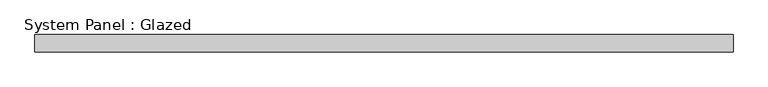
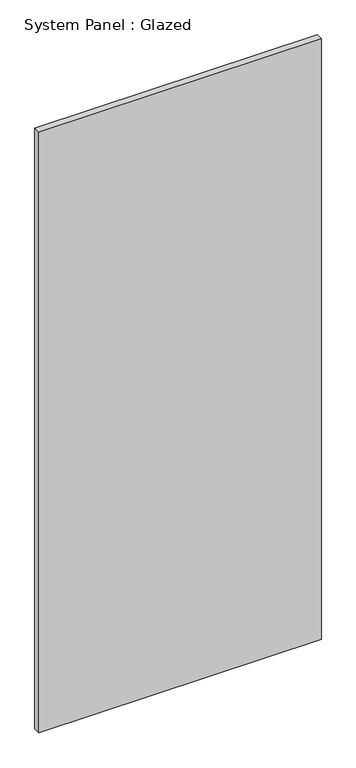
"""IFC4 building model written with IfcOpenShell, lengths in millimetres: plate geometry, System Panel : Glazed."""

from ifc_helpers import new_model, si_unit, origin, origin_with_axes, place, context, project, spatial, polyline, outline, extrude, source, transform, mapped, element, save


def system_panel_glazed_68324572(model_context):
    return source(origin(), model_context, "Body", "SweptSolid", [
        extrude(outline(polyline([(514.3499999, 19.05), (-514.3499999, 19.05), (-514.3499999, 44.45), (514.3499999, 44.45), (514.3499999, 19.05)])), origin_with_axes(), (0.0, 0.0, 1.0), 2311.4),
    ])


if __name__ == "__main__":
    model = new_model("IFC4")
    model_context = context("Model", 3, world=origin())
    ifc_project = project(units=[si_unit("LENGTHUNIT", "METRE", prefix="MILLI")], contexts=[model_context])
    site = spatial("IfcSite", under=ifc_project)
    building = spatial("IfcBuilding", under=site)
    placement = place(None, origin())
    system_panel_glazed_shape = system_panel_glazed_68324572(model_context)
    element("IfcPlate", 1, ObjectType="System Panel : Glazed", at=placement, inside=building, context=model_context, shape_type="MappedRepresentation", body=[
        mapped(system_panel_glazed_shape, transform((0.0, 0.0, 0.0), x_axis=(1.0, 0.0, 0.0), y_axis=(0.0, 1.0, 0.0), z_axis=(0.0, 0.0, 1.0))),
    ])
    save(model, "model.ifc")

# Revit data of these elements
# Type "System Panel : Glazed"
#   Construction Type Id = "GSP4R"
#   Analytic Construction = "1/8 in Pilkington single glazing"
#   Visual Light Transmittance = 0.9
#   Solar Heat Gain Coefficient = 0.86
#   Heat Transfer Coefficient (U) = 1.18115 BTU/(h·ft²·°F)
#   Define Thermal Properties by = 1
# Element 1 (IfcPlate, "System Panel : Glazed")
#   Materials on its faces: "Glass"
# Materials
#   "Glass": class "Glass", colour RGB 0 128 192, transparency 0.75, Description = "Soda Lime Glass", Cost = 0
